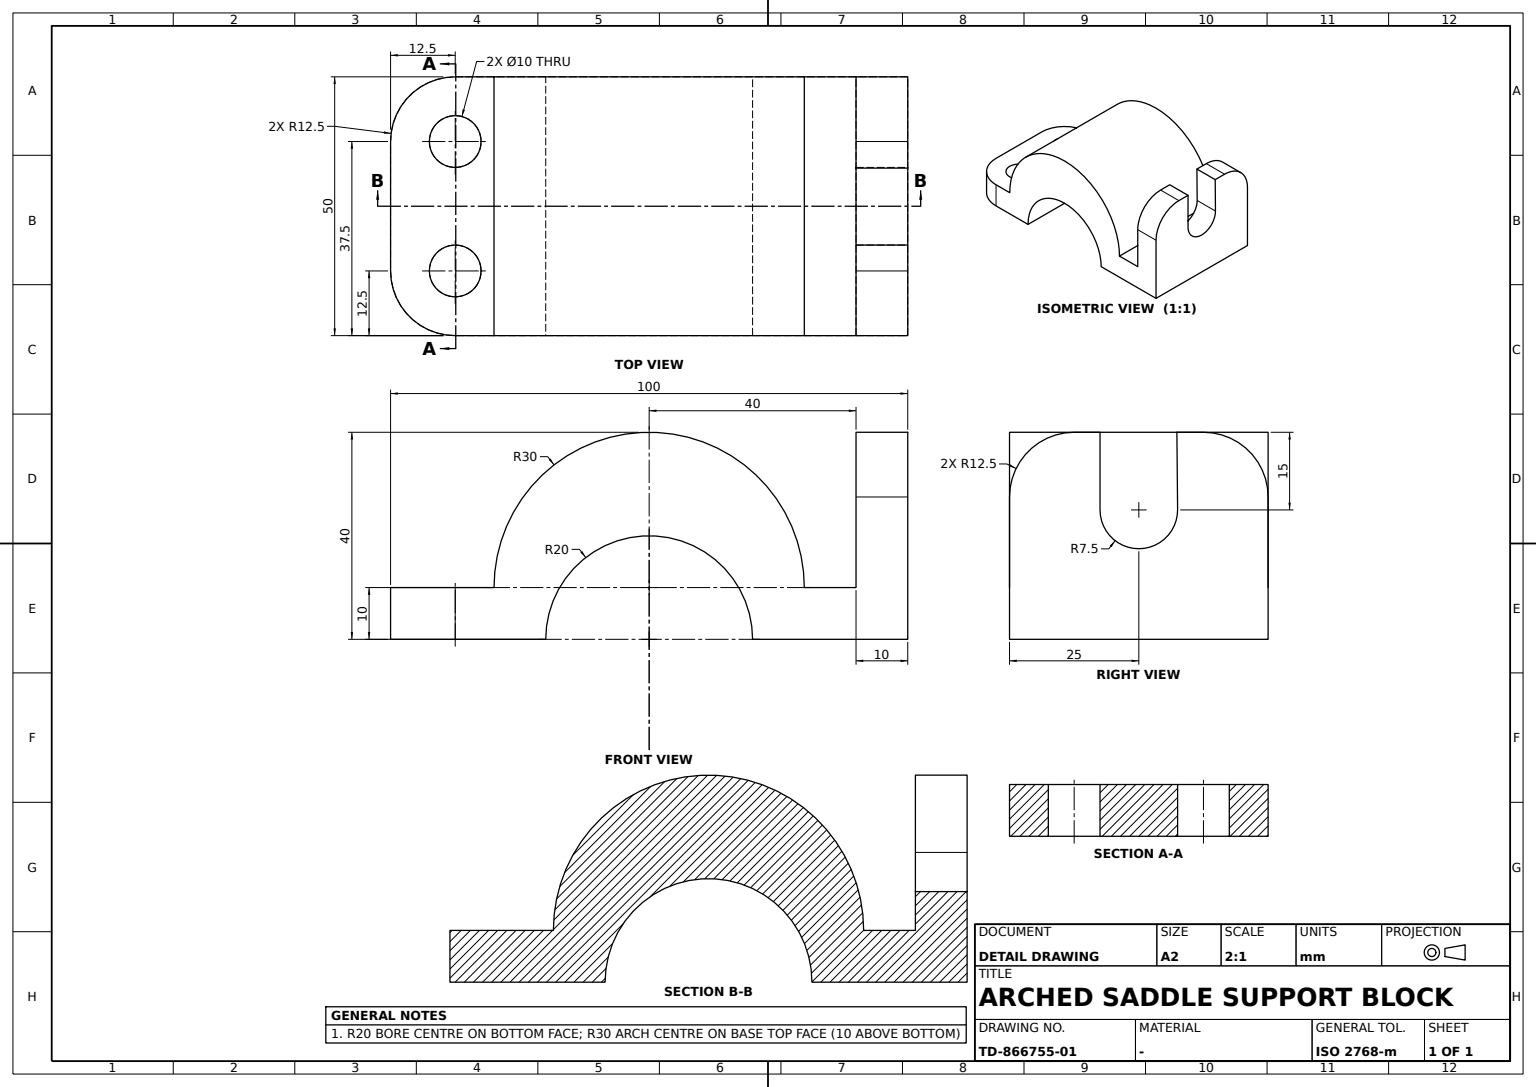
CATIA V5 part; units mm, degrees
sketch "Sketch1" plane through (0, 0, 0) normal (0, 1, 0) x (-1, 0, 0)
  line L0 (0, 0) -> (0, 40)
  line L1 (0, 40) -> (10, 40)
  line L2 (10, 40) -> (10, 10)
  line L3 (0, 0) -> (30, 0)
  point P0 (30, 0)
  arc A0 (30, 0) -> (70, 0) centre (50, 0) cw
  point P1 (30, 0)
  point P2 (70, 0)
  line L4 (10, 10) -> (20, 10)
  arc A1 (20, 10) -> (80, 10) centre (50, 10) cw
  point P3 (80, 10)
  line L5 (70, 0) -> (100, 0)
  line L6 (100, 0) -> (100, 10)
  point P4 (100, 10)
  line L7 (100, 10) -> (80, 10)
  point P5 (80, 10)
  dimension "length L1" = 10
  dimension "distance L1 L3" = 40
  dimension "length L2" = 30
  dimension "length L4" = 10
  dimension "length L3" = 30
  dimension "radius A0" = 20
  dimension "radius A1" = 30
  dimension "length L5" = 30
  dimension "length L7" = 20
  dimension "D10" = 100
  constraint vertical L0 y-axis
  constraint vertical L2 y-axis
  constraint vertical L6 y-axis
  constraint horizontal L1 x-axis
  constraint horizontal L3 x-axis
  constraint horizontal L4 x-axis
  constraint horizontal L5 x-axis
  constraint horizontal L7 x-axis
  constraint coincidence P1 L3
  constraint coincidence P2 x-axis
  constraint coincidence P1 P0
  constraint coincidence P4 L4
  constraint coincidence P5 A1
  constraint coincidence P3 P5
extrude "Pad1" add sketch "Sketch1" along normal mid plane 50
fillet "Fillet1" radius 12.5 4 edges at (-5, 25, 40) (-5, -25, 40) (-100, 25, 5) (-100, -25, 5)
sketch "Sketch2" plane through (-91.496, 17.3794, 10) normal (0, 0, 1) x (1, 0, 0)
  point P0 (3.996, -4.8794)
  point P1 (3.996, -29.8794)
  dimension "D1" = 37.5
  dimension "distance P0 P1" = 25
hole "Hole1" at (-87.5, 12.5, 10) direction (0, 0, -1) diameter 10 end up to next
mirror "Mirror1" about plane through (0, 0, 0) normal (0, 1, 0) of "Hole1"
sketch "Sketch3" plane through (0, 0, 0) normal (1, 0, 0) x (0, 1, 0)
  arc A0 (-7.5, 25) -> (7.4997, 25.0691) centre (0, 25) ccw
  point P0 (0, 25)
  line L0 (-25, 0) -> (25, 0) construction
  line L1 (-7.5, 25) -> (-7.5, 40.4757)
  line L2 (-7.5, 40.4757) -> (7.3577, 40.4757)
  line L3 (7.3577, 40.4757) -> (7.4997, 25.0691)
  dimension "radius A0" = 7.5
  dimension "distance P0 L0" = 25
  constraint coincidence P0 y-axis
  constraint tangency L1 A0
  constraint tangency L3 A0
  constraint horizontal L2 x-axis
extrude "Pocket1" cut sketch "Sketch3" against normal blind 10
properties part number "catia 12"
